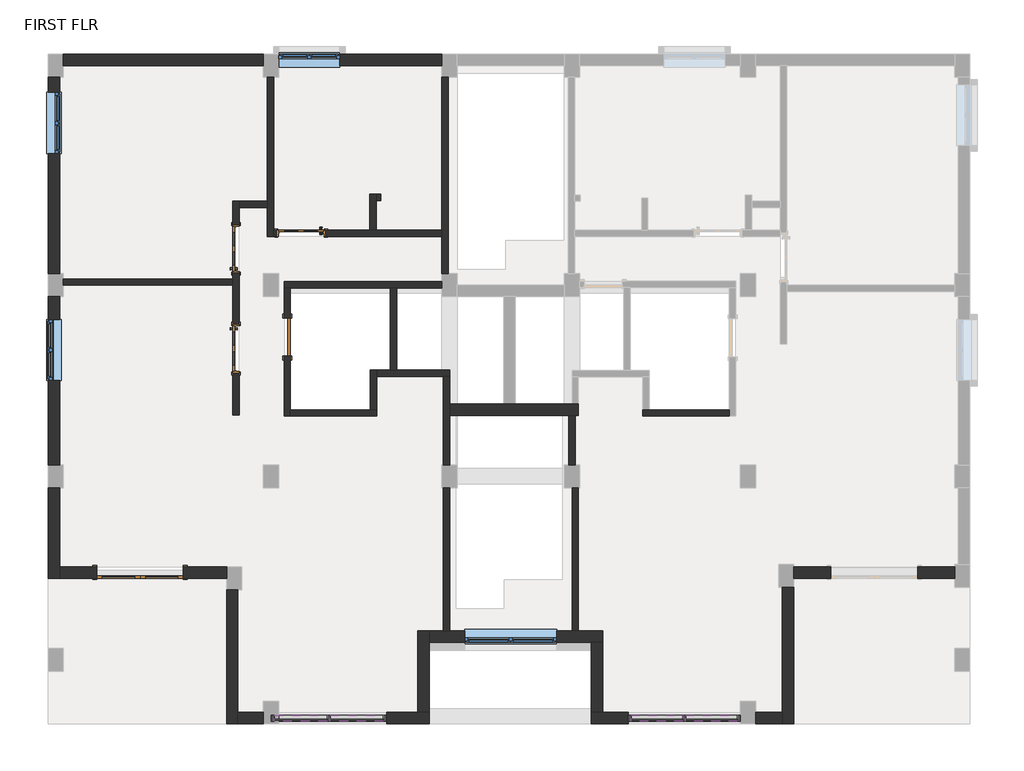
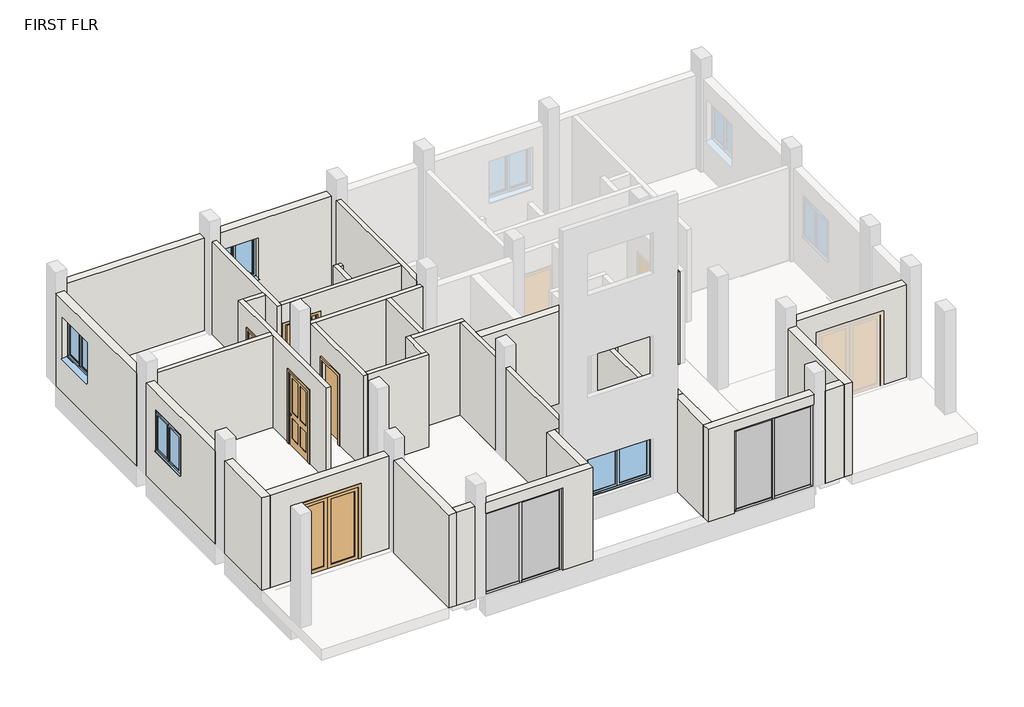
# One storey, part 1 of 3: 36 walls, 14 members, 5 doors, 4 plates, 4 windows.
"""IFC4 building model written with IfcOpenShell, lengths in millimetres."""

from ifc_helpers import new_model, si_unit, frame, origin, place, context, project, spatial, polyline, outline, extrude, faceted_brep, transform, mapped, element, save
from components import door_e52a3823, door_68a706ac, door_a823658d, door_1fe7f57d, member_a1c24a98, member_7fa39cca, member_f0fea5a5, member_ee409385, system_panel_glazed_8311221f, system_panel_glazed_a93c8db9, w2_0001_windows_4_x_4_9dec5fc7, w2_0001_window_4_x_6_83c3b52c

model = new_model("IFC4")

# Units and contexts
model_context = context("Model", 3, world=origin())
ifc_project = project(units=[si_unit("LENGTHUNIT", "METRE", prefix="MILLI")], contexts=[model_context])

# Site, building, storey
site = spatial("IfcSite", under=ifc_project)
building = spatial("IfcBuilding", under=site)
storey = spatial("IfcBuildingStorey", under=building, Name="FIRST FLR", Elevation=3352.8)

# Doors
placement = place(None, origin())
door_shape = door_e52a3823(model_context)
element("IfcDoor", 1, ObjectType="Door-Double-Glass : 68\" x 84\"", at=placement, inside=storey, context=model_context, shape_type="MappedRepresentation", body=[
    mapped(door_shape, transform((-7309.9981098, -11554.5807833, 3352.8), x_axis=(-1.0, 0.0, 0.0), y_axis=(0.0, -1.0, 0.0), z_axis=(0.0, 0.0, 1.0))),
])
door_2_shape = door_68a706ac(model_context)
element("IfcDoor", 2, ObjectType="Door-Interior-Single-4_Panel-Wood : 36\" x 84\"", at=placement, inside=storey, context=model_context, shape_type="MappedRepresentation", body=[
    mapped(door_2_shape, transform((-5402.1925798, -5105.3620333, 3352.8), x_axis=(0.0, 1.0, 0.0), y_axis=(-1.0, 0.0, 0.0), z_axis=(0.0, 0.0, 1.0))),
])
door_3_shape = door_a823658d(model_context)
element("IfcDoor", 3, ObjectType="Door-Interior-Single-4_Panel-Wood : 36\" x 84\"", at=placement, inside=storey, context=model_context, shape_type="MappedRepresentation", body=[
    mapped(door_3_shape, transform((-4103.6175798, -4789.1311634, 3352.8), x_axis=(-1.0, 0.0, 0.0), y_axis=(0.0, -1.0, 0.0), z_axis=(0.0, 0.0, 1.0))),
])
element("IfcDoor", 4, ObjectType="Door-Interior-Single-4_Panel-Wood : 36\" x 84\"", at=placement, inside=storey, context=model_context, shape_type="MappedRepresentation", body=[
    mapped(door_3_shape, transform((-5402.1925798, -7092.9120333, 3352.8), x_axis=(0.0, -1.0, 0.0), y_axis=(1.0, 0.0, 0.0), z_axis=(0.0, 0.0, 1.0))),
])
door_4_shape = door_1fe7f57d(model_context)
element("IfcDoor", 5, ObjectType="Single-Flush : 30\" x 80\"", at=placement, inside=storey, context=model_context, shape_type="MappedRepresentation", body=[
    mapped(door_4_shape, transform((-4379.0950401, -6863.7942903, 3352.8), x_axis=(0.0, -1.0, 0.0), y_axis=(1.0, 0.0, 0.0), z_axis=(0.0, 0.0, 1.0))),
])

# Members
member_shape = member_a1c24a98(model_context)
element("IfcMember", 6, ObjectType="Rectangular Mullion : 2.5\" x 5\" rectangular", at=placement, inside=storey, context=model_context, shape_type="MappedRepresentation", body=[
    mapped(member_shape, transform((2474.9824202, -14462.5402089, 5791.2), x_axis=(0.0, 0.0, 1.0), y_axis=(0.0, 1.0, 0.0), z_axis=(-1.0, 0.0, 0.0))),
])
element("IfcMember", 7, ObjectType="Rectangular Mullion : 2.5\" x 5\" rectangular", at=placement, inside=storey, context=model_context, shape_type="MappedRepresentation", body=[
    mapped(member_shape, transform((3560.8324202, -14462.5402089, 5791.2), x_axis=(0.0, 0.0, 1.0), y_axis=(0.0, 1.0, 0.0), z_axis=(-1.0, 0.0, 0.0))),
])
element("IfcMember", 8, ObjectType="Rectangular Mullion : 2.5\" x 5\" rectangular", at=placement, inside=storey, context=model_context, shape_type="MappedRepresentation", body=[
    mapped(member_shape, transform((4583.1824202, -14462.5402089, 3352.8), x_axis=(0.0, 0.0, -1.0), y_axis=(0.0, 1.0, 0.0), z_axis=(1.0, 0.0, 0.0))),
])
element("IfcMember", 9, ObjectType="Rectangular Mullion : 2.5\" x 5\" rectangular", at=placement, inside=storey, context=model_context, shape_type="MappedRepresentation", body=[
    mapped(member_shape, transform((3497.3324202, -14462.5402089, 3352.8), x_axis=(0.0, 0.0, -1.0), y_axis=(0.0, 1.0, 0.0), z_axis=(1.0, 0.0, 0.0))),
])
member_2_shape = member_7fa39cca(model_context)
element("IfcMember", 10, ObjectType="Rectangular Mullion : 2.5\" x 5\" rectangular", at=placement, inside=storey, context=model_context, shape_type="MappedRepresentation", body=[
    mapped(member_2_shape, transform((-4637.0175798, -14462.5402089, 5791.2), x_axis=(0.0, 0.0, 1.0), y_axis=(0.0, 1.0, 0.0), z_axis=(-1.0, 0.0, 0.0))),
])
element("IfcMember", 11, ObjectType="Rectangular Mullion : 2.5\" x 5\" rectangular", at=placement, inside=storey, context=model_context, shape_type="MappedRepresentation", body=[
    mapped(member_2_shape, transform((-3519.4175798, -14462.5402089, 5791.2), x_axis=(0.0, 0.0, 1.0), y_axis=(0.0, 1.0, 0.0), z_axis=(-1.0, 0.0, 0.0))),
])
element("IfcMember", 12, ObjectType="Rectangular Mullion : 2.5\" x 5\" rectangular", at=placement, inside=storey, context=model_context, shape_type="MappedRepresentation", body=[
    mapped(member_2_shape, transform((-2465.3175798, -14462.5402089, 3352.8), x_axis=(0.0, 0.0, -1.0), y_axis=(0.0, 1.0, 0.0), z_axis=(1.0, 0.0, 0.0))),
])
element("IfcMember", 13, ObjectType="Rectangular Mullion : 2.5\" x 5\" rectangular", at=placement, inside=storey, context=model_context, shape_type="MappedRepresentation", body=[
    mapped(member_2_shape, transform((-3582.9175798, -14462.5402089, 3352.8), x_axis=(0.0, 0.0, -1.0), y_axis=(0.0, 1.0, 0.0), z_axis=(1.0, 0.0, 0.0))),
])
member_3_shape = member_f0fea5a5(model_context)
element("IfcMember", 14, ObjectType="Rectangular Mullion : 2.5\" x 5\" rectangular", at=placement, inside=storey, context=model_context, shape_type="MappedRepresentation", body=[
    mapped(member_3_shape, transform((3529.0824202, -14462.5402089, 3352.8), x_axis=(-1.0, 0.0, 0.0), y_axis=(0.0, 1.0, 0.0), z_axis=(0.0, 0.0, -1.0))),
])
element("IfcMember", 15, ObjectType="Rectangular Mullion : 2.5\" x 5\" rectangular", at=placement, inside=storey, context=model_context, shape_type="MappedRepresentation", body=[
    mapped(member_3_shape, transform((-3551.1675798, -14462.5402089, 3352.8), x_axis=(-1.0, 0.0, 0.0), y_axis=(0.0, 1.0, 0.0), z_axis=(0.0, 0.0, -1.0))),
])
member_4_shape = member_ee409385(model_context)
element("IfcMember", 16, ObjectType="Rectangular Mullion : 2.5\" x 5\" rectangular", at=placement, inside=storey, context=model_context, shape_type="MappedRepresentation", body=[
    mapped(member_4_shape, transform((2411.4824202, -14462.5402089, 3352.8), x_axis=(-1.0, 0.0, 0.0), y_axis=(0.0, 1.0, 0.0), z_axis=(0.0, 0.0, -1.0))),
])
element("IfcMember", 17, ObjectType="Rectangular Mullion : 2.5\" x 5\" rectangular", at=placement, inside=storey, context=model_context, shape_type="MappedRepresentation", body=[
    mapped(member_4_shape, transform((-4700.5175798, -14462.5402089, 3352.8), x_axis=(-1.0, 0.0, 0.0), y_axis=(0.0, 1.0, 0.0), z_axis=(0.0, 0.0, -1.0))),
])
element("IfcMember", 18, ObjectType="Rectangular Mullion : 2.5\" x 5\" rectangular", at=placement, inside=storey, context=model_context, shape_type="MappedRepresentation", body=[
    mapped(member_4_shape, transform((4646.6824202, -14462.5402089, 5791.2), x_axis=(1.0, 0.0, 0.0), y_axis=(0.0, 1.0, 0.0), z_axis=(0.0, 0.0, 1.0))),
])
element("IfcMember", 19, ObjectType="Rectangular Mullion : 2.5\" x 5\" rectangular", at=placement, inside=storey, context=model_context, shape_type="MappedRepresentation", body=[
    mapped(member_4_shape, transform((-2401.8175798, -14462.5402089, 5791.2), x_axis=(1.0, 0.0, 0.0), y_axis=(0.0, 1.0, 0.0), z_axis=(0.0, 0.0, 1.0))),
])

# Plates
system_panel_glazed_shape = system_panel_glazed_8311221f(model_context)
element("IfcPlate", 20, ObjectType="System Panel : Glazed", at=placement, inside=storey, context=model_context, shape_type="MappedRepresentation", body=[
    mapped(system_panel_glazed_shape, transform((4072.0074202, -14462.5402089, 3416.3), x_axis=(-1.0, 0.0, 0.0), y_axis=(0.0, -1.0, 0.0), z_axis=(0.0, 0.0, 1.0))),
])
element("IfcPlate", 21, ObjectType="System Panel : Glazed", at=placement, inside=storey, context=model_context, shape_type="MappedRepresentation", body=[
    mapped(system_panel_glazed_shape, transform((2986.1574202, -14462.5402089, 3416.3), x_axis=(-1.0, 0.0, 0.0), y_axis=(0.0, -1.0, 0.0), z_axis=(0.0, 0.0, 1.0))),
])
system_panel_glazed_2_shape = system_panel_glazed_a93c8db9(model_context)
element("IfcPlate", 22, ObjectType="System Panel : Glazed", at=placement, inside=storey, context=model_context, shape_type="MappedRepresentation", body=[
    mapped(system_panel_glazed_2_shape, transform((-2992.3675798, -14462.5402089, 3416.3), x_axis=(-1.0, 0.0, 0.0), y_axis=(0.0, -1.0, 0.0), z_axis=(0.0, 0.0, 1.0))),
])
element("IfcPlate", 23, ObjectType="System Panel : Glazed", at=placement, inside=storey, context=model_context, shape_type="MappedRepresentation", body=[
    mapped(system_panel_glazed_2_shape, transform((-4109.9675798, -14462.5402089, 3416.3), x_axis=(-1.0, 0.0, 0.0), y_axis=(0.0, -1.0, 0.0), z_axis=(0.0, 0.0, 1.0))),
])

# Walls
element("IfcWall", 24, ObjectType="EXTERIOR WALL 9\"", at=placement, inside=storey, context=model_context, shape_type="SweptSolid", body=[
    extrude(outline(polyline([(-4852.9175798, -1452.2061634), (-8839.9786397, -1452.2061634), (-8839.9786397, -1223.6061634), (-4852.9175798, -1223.6061634), (-4852.9175798, -1452.2061634)])), frame((0.0, 0.0, 3352.8), z_axis=(0.0, 0.0, 1.0), x_axis=(1.0, 0.0, 0.0)), (0.0, 0.0, 1.0), 2743.2),
])
element("IfcWall", 25, ObjectType="EXTERIOR WALL 9\"", at=placement, inside=storey, context=model_context, shape_type="SweptSolid", body=[
    extrude(outline(polyline([(4352.8, -3328.9175798), (4352.8, -4548.1175798), (3352.8, -4548.1175798), (3352.8, -1296.9175798), (6096.0, -1296.9175798), (6096.0, -4548.1175798), (5572.0, -4548.1175798), (5572.0, -3328.9175798), (4352.8, -3328.9175798)])), frame((0.0, -1452.2061634, 0.0), z_axis=(0.0, 1.0, 0.0), x_axis=(0.0, 0.0, 1.0)), (0.0, 0.0, 1.0), 228.6),
])
element("IfcWall", 26, ObjectType="EXTERIOR WALL 9\"", at=placement, inside=storey, context=model_context, shape_type="SweptSolid", body=[
    extrude(outline(polyline([(-1680.8061634, 3352.8), (-5600.6620333, 3352.8), (-5600.6620333, 6096.0), (-1680.8061634, 6096.0), (-1680.8061634, 3352.8)]), holes=[polyline([(-3204.8061634, 4352.8), (-1985.6061634, 4352.8), (-1985.6061634, 5572.0), (-3204.8061634, 5572.0), (-3204.8061634, 4352.8)])]), frame((-9144.7786397, 0.0, 0.0), z_axis=(1.0, 0.0, 0.0), x_axis=(0.0, 1.0, 0.0)), (0.0, 0.0, 1.0), 228.6),
])
element("IfcWall", 27, ObjectType="EXTERIOR WALL 9\"", at=placement, inside=storey, context=model_context, shape_type="SweptSolid", body=[
    extrude(outline(polyline([(-6057.8620333, 3352.8), (-9410.6620333, 3352.8), (-9410.6620333, 6096.0), (-6057.8620333, 6096.0), (-6057.8620333, 3352.8)]), holes=[polyline([(-6515.0620333, 4352.8), (-6515.0620333, 5572.0), (-7734.2620333, 5572.0), (-7734.2620333, 4352.8), (-6515.0620333, 4352.8)])]), frame((-9144.7786397, 0.0, 0.0), z_axis=(1.0, 0.0, 0.0), x_axis=(0.0, 1.0, 0.0)), (0.0, 0.0, 1.0), 228.6),
])
element("IfcWall", 28, ObjectType="EXTERIOR WALL 9\"", at=placement, inside=storey, context=model_context, shape_type="Brep", body=[
    faceted_brep([(-9144.7786397, -9867.8620333, 3352.8), (-9144.7786397, -11671.2620333, 3352.8), (-9144.7786397, -11671.2620333, 6096.0), (-9144.7786397, -9867.8620333, 6096.0), (-8916.1786397, -9867.8620333, 3352.8), (-8916.1786397, -9867.8620333, 6096.0), (-8916.1786397, -11442.6620333, 6096.0), (-8916.1786397, -11671.2620333, 6096.0), (-8916.1786397, -11671.2620333, 3352.8), (-8916.1786397, -11442.6620333, 3352.8)], [[[0, 1, 2, 3]], [[4, 5, 6, 7, 8, 9]], [[1, 0, 4, 9, 8]], [[3, 2, 7, 6, 5]], [[0, 3, 5, 4]], [[2, 1, 8, 7]]]),
])
element("IfcWall", 29, ObjectType="EXTERIOR WALL 9\"", at=placement, inside=storey, context=model_context, shape_type="SweptSolid", body=[
    extrude(outline(polyline([(6096.0, -5589.5175798), (6096.0, -8916.1786397), (3352.8, -8916.1786397), (3352.8, -8173.5981098), (5486.4, -8173.5981098), (5486.4, -6446.3981098), (3352.8, -6446.3981098), (3352.8, -5589.5175798), (6096.0, -5589.5175798)])), frame((0.0, -11671.2620333, 0.0), z_axis=(0.0, 1.0, 0.0), x_axis=(0.0, 0.0, 1.0)), (0.0, 0.0, 1.0), 228.6),
])
element("IfcWall", 30, ObjectType="EXTERIOR WALL 9\"", at=placement, inside=storey, context=model_context, shape_type="SweptSolid", body=[
    extrude(outline(polyline([(6096.0, 5713.4824202), (3352.8, 5713.4824202), (3352.8, 6450.0824202), (5486.4, 6450.0824202), (5486.4, 8177.2824202), (3352.8, 8177.2824202), (3352.8, 8913.8824202), (6096.0, 8913.8824202), (6096.0, 5713.4824202)])), frame((0.0, -11671.2620333, 0.0), z_axis=(0.0, 1.0, 0.0), x_axis=(0.0, 0.0, 1.0)), (0.0, 0.0, 1.0), 228.6),
])
element("IfcWall", 31, ObjectType="EXTERIOR WALL 9\"", at=placement, inside=storey, context=model_context, shape_type="Brep", body=[
    faceted_brep([(5484.8824202, -11849.0620333, 3352.8), (5484.8824202, -14348.2402089, 3352.8), (5484.8824202, -14576.8402089, 3352.8), (5484.8824202, -14576.8402089, 6096.0), (5484.8824202, -14348.2402089, 6096.0), (5484.8824202, -11849.0620333, 6096.0), (5713.4824202, -11849.0620333, 3352.8), (5713.4824202, -11849.0620333, 6096.0), (5713.4824202, -14576.8402089, 6096.0), (5713.4824202, -14576.8402089, 3352.8)], [[[0, 1, 2, 3, 4, 5]], [[6, 7, 8, 9]], [[2, 1, 0, 6, 9]], [[5, 4, 3, 8, 7]], [[0, 5, 7, 6]], [[3, 2, 9, 8]]]),
])
element("IfcWall", 32, ObjectType="EXTERIOR WALL 9\"", at=placement, inside=storey, context=model_context, shape_type="SweptSolid", body=[
    extrude(outline(polyline([(5484.8824202, -14576.8402089), (4951.4824202, -14576.8402089), (4951.4824202, -14348.2402089), (5484.8824202, -14348.2402089), (5484.8824202, -14576.8402089)])), frame((0.0, 0.0, 3352.8), z_axis=(0.0, 0.0, 1.0), x_axis=(1.0, 0.0, 0.0)), (0.0, 0.0, 1.0), 2743.2),
])
element("IfcWall", 33, ObjectType="EXTERIOR WALL 9\"", at=placement, inside=storey, context=model_context, shape_type="Brep", body=[
    faceted_brep([(-5589.5175798, -11899.8620333, 3352.8), (-5589.5175798, -14576.8402089, 3352.8), (-5589.5175798, -14576.8402089, 6096.0), (-5589.5175798, -11899.8620333, 6096.0), (-5360.9175798, -11899.8620333, 3352.8), (-5360.9175798, -11899.8620333, 6096.0), (-5360.9175798, -14348.2402089, 6096.0), (-5360.9175798, -14576.8402089, 6096.0), (-5360.9175798, -14576.8402089, 3352.8), (-5360.9175798, -14348.2402089, 3352.8)], [[[0, 1, 2, 3]], [[4, 5, 6, 7, 8, 9]], [[1, 0, 4, 9, 8]], [[3, 2, 7, 6, 5]], [[0, 3, 5, 4]], [[2, 1, 8, 7]]]),
])
element("IfcWall", 34, ObjectType="EXTERIOR WALL 9\"", at=placement, inside=storey, context=model_context, shape_type="SweptSolid", body=[
    extrude(outline(polyline([(-5360.9175798, -14348.2402089), (-4852.9175798, -14348.2402089), (-4852.9175798, -14576.8402089), (-5360.9175798, -14576.8402089), (-5360.9175798, -14348.2402089)])), frame((0.0, 0.0, 3352.8), z_axis=(0.0, 0.0, 1.0), x_axis=(1.0, 0.0, 0.0)), (0.0, 0.0, 1.0), 2743.2),
])
element("IfcWall", 35, ObjectType="EXTERIOR WALL 9\"", at=placement, inside=storey, context=model_context, shape_type="Brep", body=[
    faceted_brep([(1674.8824202, -14348.2402089, 6096.0), (1903.4824202, -14348.2402089, 6096.0), (4646.6824202, -14348.2402089, 6096.0), (4646.6824202, -14348.2402089, 5791.2), (2411.4824202, -14348.2402089, 5791.2), (2411.4824202, -14348.2402089, 3352.8), (1903.4824202, -14348.2402089, 3352.8), (1674.8824202, -14348.2402089, 3352.8), (4646.6824202, -14576.8402089, 6096.0), (1674.8824202, -14576.8402089, 6096.0), (1674.8824202, -14576.8402089, 3352.8), (2411.4824202, -14576.8402089, 3352.8), (2411.4824202, -14576.8402089, 5791.2), (4646.6824202, -14576.8402089, 5791.2)], [[[0, 1, 2, 3, 4, 5, 6, 7]], [[8, 9, 10, 11, 12, 13]], [[10, 7, 6, 5, 11]], [[2, 1, 0, 9, 8]], [[2, 8, 13, 3]], [[0, 7, 10, 9]], [[4, 12, 11, 5]], [[12, 4, 3, 13]]]),
])
element("IfcWall", 36, ObjectType="EXTERIOR WALL 9\"", at=placement, inside=storey, context=model_context, shape_type="Brep", body=[
    faceted_brep([(-1550.9175798, -14576.8402089, 6096.0), (-4548.1175798, -14576.8402089, 6096.0), (-4548.1175798, -14576.8402089, 5791.2), (-2401.8175798, -14576.8402089, 5791.2), (-2401.8175798, -14576.8402089, 3352.8), (-1550.9175798, -14576.8402089, 3352.8), (-4548.1175798, -14348.2402089, 6096.0), (-1779.5175798, -14348.2402089, 6096.0), (-1550.9175798, -14348.2402089, 6096.0), (-1550.9175798, -14348.2402089, 3352.8), (-1779.5175798, -14348.2402089, 3352.8), (-2401.8175798, -14348.2402089, 3352.8), (-2401.8175798, -14348.2402089, 5791.2), (-4548.1175798, -14348.2402089, 5791.2)], [[[0, 1, 2, 3, 4, 5]], [[6, 7, 8, 9, 10, 11, 12, 13]], [[9, 5, 4, 11, 10]], [[1, 0, 8, 7, 6]], [[1, 6, 13, 2]], [[0, 5, 9, 8]], [[3, 12, 11, 4]], [[12, 3, 2, 13]]]),
])
element("IfcWall", 37, ObjectType="EXTERIOR WALL 9\"", at=placement, inside=storey, context=model_context, shape_type="Brep", body=[
    faceted_brep([(-1550.9175798, -14348.2402089, 3352.8), (-1550.9175798, -12951.2402089, 3352.8), (-1550.9175798, -12722.6402089, 3352.8), (-1550.9175798, -12722.6402089, 6096.0), (-1550.9175798, -12951.2402089, 6096.0), (-1550.9175798, -14348.2402089, 6096.0), (-1779.5175798, -14348.2402089, 3352.8), (-1779.5175798, -14348.2402089, 6096.0), (-1779.5175798, -12722.6402089, 6096.0), (-1779.5175798, -12722.6402089, 3352.8)], [[[0, 1, 2, 3, 4, 5]], [[6, 7, 8, 9]], [[2, 1, 0, 6, 9]], [[5, 4, 3, 8, 7]], [[0, 5, 7, 6]], [[3, 2, 9, 8]]]),
])
element("IfcWall", 38, ObjectType="EXTERIOR WALL 9\"", at=placement, inside=storey, context=model_context, shape_type="Brep", body=[
    faceted_brep([(-1550.9175798, -12951.2402089, 3352.8), (1674.8824202, -12951.2402089, 3352.8), (1903.4824202, -12951.2402089, 3352.8), (1903.4824202, -12951.2402089, 6096.0), (1674.8824202, -12951.2402089, 6096.0), (-1550.9175798, -12951.2402089, 6096.0), (-839.7175798, -12951.2402089, 3962.4), (-839.7175798, -12951.2402089, 5181.6), (989.0824202, -12951.2402089, 5181.6), (989.0824202, -12951.2402089, 3962.4), (-1550.9175798, -12722.6402089, 3352.8), (-1550.9175798, -12722.6402089, 6096.0), (-1271.5175798, -12722.6402089, 6096.0), (-1144.5175798, -12722.6402089, 6096.0), (1293.8824202, -12722.6402089, 6096.0), (1420.8824202, -12722.6402089, 6096.0), (1903.4824202, -12722.6402089, 6096.0), (1903.4824202, -12722.6402089, 3352.8), (1420.8824202, -12722.6402089, 3352.8), (1293.8824202, -12722.6402089, 3352.8), (-1144.5175798, -12722.6402089, 3352.8), (-1271.5175798, -12722.6402089, 3352.8), (-839.7175798, -12722.6402089, 3962.4), (989.0824202, -12722.6402089, 3962.4), (989.0824202, -12722.6402089, 5181.6), (-839.7175798, -12722.6402089, 5181.6)], [[[0, 1, 2, 3, 4, 5], [6, 7, 8, 9]], [[10, 11, 12, 13, 14, 15, 16, 17, 18, 19, 20, 21], [22, 23, 24, 25]], [[2, 1, 0, 10, 21, 20, 19, 18, 17]], [[5, 4, 3, 16, 15, 14, 13, 12, 11]], [[0, 5, 11, 10]], [[3, 2, 17, 16]], [[7, 6, 22, 25]], [[8, 7, 25, 24]], [[9, 8, 24, 23]], [[6, 9, 23, 22]]]),
])
element("IfcWall", 39, ObjectType="EXTERIOR WALL 9\"", at=placement, inside=storey, context=model_context, shape_type="SweptSolid", body=[
    extrude(outline(polyline([(1674.8824202, -14348.2402089), (1674.8824202, -12951.2402089), (1903.4824202, -12951.2402089), (1903.4824202, -14348.2402089), (1674.8824202, -14348.2402089)])), frame((0.0, 0.0, 3352.8), z_axis=(0.0, 0.0, 1.0), x_axis=(1.0, 0.0, 0.0)), (0.0, 0.0, 1.0), 2743.2),
])
element("IfcWall", 40, ObjectType="EXTERIOR WALL 9\"", at=placement, inside=storey, context=model_context, shape_type="Brep", body=[
    faceted_brep([(-1144.5175798, -8426.4120333, 3352.8), (1230.3824202, -8426.4120333, 3352.8), (1357.3824202, -8426.4120333, 3352.8), (1420.8824202, -8426.4120333, 3352.8), (1420.8824202, -8426.4120333, 6096.0), (1357.3824202, -8426.4120333, 6096.0), (1230.3824202, -8426.4120333, 6096.0), (-1144.5175798, -8426.4120333, 6096.0), (-1144.5175798, -8197.8120333, 3352.8), (-1144.5175798, -8197.8120333, 6096.0), (-65.0175798, -8197.8120333, 6096.0), (163.5824202, -8197.8120333, 6096.0), (1293.8824202, -8197.8120333, 6096.0), (1420.8824202, -8197.8120333, 6096.0), (1420.8824202, -8197.8120333, 3352.8), (1293.8824202, -8197.8120333, 3352.8), (163.5824202, -8197.8120333, 3352.8), (-65.0175798, -8197.8120333, 3352.8)], [[[0, 1, 2, 3, 4, 5, 6, 7]], [[8, 9, 10, 11, 12, 13, 14, 15, 16, 17]], [[3, 2, 1, 0, 8, 17, 16, 15, 14]], [[7, 6, 5, 4, 13, 12, 11, 10, 9]], [[0, 7, 9, 8]], [[4, 3, 14, 13]]]),
])
element("IfcWall", 41, ObjectType="INTERIOR WALL 5\"", at=placement, inside=storey, context=model_context, shape_type="SweptSolid", body=[
    extrude(outline(polyline([(-5462.5175798, -5829.2620333), (-8839.9786397, -5829.2620333), (-8839.9786397, -5702.2620333), (-5462.5175798, -5702.2620333), (-5462.5175798, -5829.2620333)])), frame((0.0, 0.0, 3352.8), z_axis=(0.0, 0.0, 1.0), x_axis=(1.0, 0.0, 0.0)), (0.0, 0.0, 1.0), 2743.2),
])
element("IfcWall", 42, ObjectType="INTERIOR WALL 5\"", at=placement, inside=storey, context=model_context, shape_type="Brep", body=[
    faceted_brep([(-5462.5175798, -8420.0620333, 3352.8), (-5462.5175798, -8420.0620333, 6096.0), (-5462.5175798, -5829.2620333, 6096.0), (-5462.5175798, -5702.2620333, 6096.0), (-5462.5175798, -4153.3104011, 6096.0), (-5462.5175798, -4153.3104011, 3352.8), (-5462.5175798, -4622.7620333, 3352.8), (-5462.5175798, -4622.7620333, 5511.8), (-5462.5175798, -5587.9620333, 5511.8), (-5462.5175798, -5587.9620333, 3352.8), (-5462.5175798, -5702.2620333, 3352.8), (-5462.5175798, -5829.2620333, 3352.8), (-5462.5175798, -6610.3120333, 3352.8), (-5462.5175798, -6610.3120333, 5511.8), (-5462.5175798, -7575.5120333, 5511.8), (-5462.5175798, -7575.5120333, 3352.8), (-5335.5175798, -8420.0620333, 6096.0), (-5335.5175798, -8420.0620333, 3352.8), (-5335.5175798, -7575.5120333, 3352.8), (-5335.5175798, -7575.5120333, 5511.8), (-5335.5175798, -6610.3120333, 5511.8), (-5335.5175798, -6610.3120333, 3352.8), (-5335.5175798, -5587.9620333, 3352.8), (-5335.5175798, -5587.9620333, 5511.8), (-5335.5175798, -4622.7620333, 5511.8), (-5335.5175798, -4622.7620333, 3352.8), (-5335.5175798, -4280.3104011, 3352.8), (-5335.5175798, -4153.3104011, 3352.8), (-5335.5175798, -4153.3104011, 6096.0), (-5335.5175798, -4280.3104011, 6096.0)], [[[0, 1, 2, 3, 4, 5, 6, 7, 8, 9, 10, 11, 12, 13, 14, 15]], [[16, 17, 18, 19, 20, 21, 22, 23, 24, 25, 26, 27, 28, 29]], [[17, 0, 15, 18]], [[5, 27, 26, 25, 6]], [[9, 22, 21, 12, 11, 10]], [[1, 0, 17, 16]], [[4, 3, 2, 1, 16, 29, 28]], [[5, 4, 28, 27]], [[24, 7, 6, 25]], [[7, 24, 23, 8]], [[8, 23, 22, 9]], [[14, 19, 18, 15]], [[19, 14, 13, 20]], [[20, 13, 12, 21]]]),
])
element("IfcWall", 43, ObjectType="INTERIOR WALL 5\"", at=placement, inside=storey, context=model_context, shape_type="SweptSolid", body=[
    extrude(outline(polyline([(-4776.7175798, -4280.3104011), (-5335.5175798, -4280.3104011), (-5335.5175798, -4153.3104011), (-4776.7175798, -4153.3104011), (-4776.7175798, -4280.3104011)])), frame((0.0, 0.0, 3352.8), z_axis=(0.0, 0.0, 1.0), x_axis=(1.0, 0.0, 0.0)), (0.0, 0.0, 1.0), 2743.2),
])
element("IfcWall", 44, ObjectType="INTERIOR WALL 5\"", at=placement, inside=storey, context=model_context, shape_type="Brep", body=[
    faceted_brep([(-4776.7175798, -1680.8061634, 3352.8), (-4776.7175798, -4153.3104011, 3352.8), (-4776.7175798, -4280.3104011, 3352.8), (-4776.7175798, -4855.8061634, 3352.8), (-4776.7175798, -4855.8061634, 6096.0), (-4776.7175798, -4280.3104011, 6096.0), (-4776.7175798, -4153.3104011, 6096.0), (-4776.7175798, -1680.8061634, 6096.0), (-4649.7175798, -1680.8061634, 3352.8), (-4649.7175798, -1680.8061634, 6096.0), (-4649.7175798, -4728.8061634, 6096.0), (-4649.7175798, -4855.8061634, 6096.0), (-4649.7175798, -4855.8061634, 3352.8), (-4649.7175798, -4728.8061634, 3352.8)], [[[0, 1, 2, 3, 4, 5, 6, 7]], [[8, 9, 10, 11, 12, 13]], [[3, 2, 1, 0, 8, 13, 12]], [[7, 6, 5, 4, 11, 10, 9]], [[0, 7, 9, 8]], [[4, 3, 12, 11]]]),
])
element("IfcWall", 45, ObjectType="INTERIOR WALL 5\"", at=placement, inside=storey, context=model_context, shape_type="Brep", body=[
    faceted_brep([(-1296.9175798, -4855.8061634, 6096.0), (-4649.7175798, -4855.8061634, 6096.0), (-4649.7175798, -4855.8061634, 3352.8), (-4586.2175798, -4855.8061634, 3352.8), (-4586.2175798, -4855.8061634, 5511.8), (-3621.0175798, -4855.8061634, 5511.8), (-3621.0175798, -4855.8061634, 3352.8), (-1296.9175798, -4855.8061634, 3352.8), (-4649.7175798, -4728.8061634, 6096.0), (-2732.0175798, -4728.8061634, 6096.0), (-2605.0175798, -4728.8061634, 6096.0), (-1296.9175798, -4728.8061634, 6096.0), (-1296.9175798, -4728.8061634, 3352.8), (-2605.0175798, -4728.8061634, 3352.8), (-2732.0175798, -4728.8061634, 3352.8), (-3621.0175798, -4728.8061634, 3352.8), (-3621.0175798, -4728.8061634, 5511.8), (-4586.2175798, -4728.8061634, 5511.8), (-4586.2175798, -4728.8061634, 3352.8), (-4649.7175798, -4728.8061634, 3352.8)], [[[0, 1, 2, 3, 4, 5, 6, 7]], [[8, 9, 10, 11, 12, 13, 14, 15, 16, 17, 18, 19]], [[2, 19, 18, 3]], [[12, 7, 6, 15, 14, 13]], [[1, 0, 11, 10, 9, 8]], [[2, 1, 8, 19]], [[0, 7, 12, 11]], [[17, 4, 3, 18]], [[4, 17, 16, 5]], [[5, 16, 15, 6]]]),
])
element("IfcWall", 46, ObjectType="INTERIOR WALL 5\"", at=placement, inside=storey, context=model_context, shape_type="Brep", body=[
    faceted_brep([(-1296.9175798, -1680.8061634, 3352.8), (-1296.9175798, -4728.8061634, 3352.8), (-1296.9175798, -4855.8061634, 3352.8), (-1296.9175798, -5600.6620333, 3352.8), (-1296.9175798, -5600.6620333, 6096.0), (-1296.9175798, -4855.8061634, 6096.0), (-1296.9175798, -4728.8061634, 6096.0), (-1296.9175798, -1680.8061634, 6096.0), (-1169.9175798, -1680.8061634, 3352.8), (-1169.9175798, -1680.8061634, 6096.0), (-1169.9175798, -5600.6620333, 6096.0), (-1169.9175798, -5600.6620333, 3352.8)], [[[0, 1, 2, 3, 4, 5, 6, 7]], [[8, 9, 10, 11]], [[3, 2, 1, 0, 8, 11]], [[4, 3, 11, 10]], [[7, 6, 5, 4, 10, 9]], [[0, 7, 9, 8]]]),
])
element("IfcWall", 47, ObjectType="INTERIOR WALL 5\"", at=placement, inside=storey, context=model_context, shape_type="Brep", body=[
    faceted_brep([(-2605.0175798, -4728.8061634, 3352.8), (-2605.0175798, -4144.6061634, 3352.8), (-2605.0175798, -4017.6061634, 3352.8), (-2605.0175798, -4017.6061634, 6096.0), (-2605.0175798, -4144.6061634, 6096.0), (-2605.0175798, -4728.8061634, 6096.0), (-2732.0175798, -4728.8061634, 3352.8), (-2732.0175798, -4728.8061634, 6096.0), (-2732.0175798, -4017.6061634, 6096.0), (-2732.0175798, -4017.6061634, 3352.8)], [[[0, 1, 2, 3, 4, 5]], [[6, 7, 8, 9]], [[2, 1, 0, 6, 9]], [[5, 4, 3, 8, 7]], [[0, 5, 7, 6]], [[3, 2, 9, 8]]]),
])
element("IfcWall", 48, ObjectType="INTERIOR WALL 5\"", at=placement, inside=storey, context=model_context, shape_type="SweptSolid", body=[
    extrude(outline(polyline([(-2605.0175798, -4017.6061634), (-2516.1175798, -4017.6061634), (-2516.1175798, -4144.6061634), (-2605.0175798, -4144.6061634), (-2605.0175798, -4017.6061634)])), frame((0.0, 0.0, 3352.8), z_axis=(0.0, 0.0, 1.0), x_axis=(1.0, 0.0, 0.0)), (0.0, 0.0, 1.0), 2743.2),
])
element("IfcWall", 49, ObjectType="INTERIOR WALL 5\"", at=placement, inside=storey, context=model_context, shape_type="Brep", body=[
    faceted_brep([(-4442.5950401, -5885.8942903, 3352.8), (-4315.5950401, -5885.8942903, 3352.8), (-2325.6175798, -5885.8942903, 3352.8), (-2198.6175798, -5885.8942903, 3352.8), (-1296.9175798, -5885.8942903, 3352.8), (-1296.9175798, -5885.8942903, 6096.0), (-2198.6175798, -5885.8942903, 6096.0), (-2325.6175798, -5885.8942903, 6096.0), (-4315.5950401, -5885.8942903, 6096.0), (-4442.5950401, -5885.8942903, 6096.0), (-4442.5950401, -5758.8942903, 3352.8), (-4442.5950401, -5758.8942903, 6096.0), (-1296.9175798, -5758.8942903, 6096.0), (-1296.9175798, -5758.8942903, 3352.8)], [[[0, 1, 2, 3, 4, 5, 6, 7, 8, 9]], [[10, 11, 12, 13]], [[4, 3, 2, 1, 0, 10, 13]], [[5, 4, 13, 12]], [[9, 8, 7, 6, 5, 12, 11]], [[0, 9, 11, 10]]]),
])
element("IfcWall", 50, ObjectType="INTERIOR WALL 5\"", at=placement, inside=storey, context=model_context, shape_type="Brep", body=[
    faceted_brep([(-4442.5950401, -7244.7942903, 5384.8), (-4442.5950401, -7244.7942903, 3352.8), (-4442.5950401, -8439.1120333, 3352.8), (-4442.5950401, -8439.1120333, 6096.0), (-4442.5950401, -5885.8942903, 6096.0), (-4442.5950401, -5885.8942903, 3352.8), (-4442.5950401, -6482.7942903, 3352.8), (-4442.5950401, -6482.7942903, 5384.8), (-4315.5950401, -8439.1120333, 3352.8), (-4315.5950401, -8312.1120333, 3352.8), (-4315.5950401, -7244.7942903, 3352.8), (-4315.5950401, -7244.7942903, 5384.8), (-4315.5950401, -6482.7942903, 5384.8), (-4315.5950401, -6482.7942903, 3352.8), (-4315.5950401, -5885.8942903, 3352.8), (-4315.5950401, -5885.8942903, 6096.0), (-4315.5950401, -8312.1120333, 6096.0), (-4315.5950401, -8439.1120333, 6096.0)], [[[0, 1, 2, 3, 4, 5, 6, 7]], [[8, 9, 10, 11, 12, 13, 14, 15, 16, 17]], [[6, 5, 14, 13]], [[2, 1, 10, 9, 8]], [[4, 3, 17, 16, 15]], [[5, 4, 15, 14]], [[3, 2, 8, 17]], [[11, 10, 1, 0]], [[12, 11, 0, 7]], [[13, 12, 7, 6]]]),
])
element("IfcWall", 51, ObjectType="INTERIOR WALL 5\"", at=placement, inside=storey, context=model_context, shape_type="Brep", body=[
    faceted_brep([(-4315.5950401, -8439.1120333, 3352.8), (-2601.0950401, -8439.1120333, 3352.8), (-2601.0950401, -8439.1120333, 6096.0), (-4315.5950401, -8439.1120333, 6096.0), (-4315.5950401, -8312.1120333, 3352.8), (-4315.5950401, -8312.1120333, 6096.0), (-2728.0950401, -8312.1120333, 6096.0), (-2601.0950401, -8312.1120333, 6096.0), (-2601.0950401, -8312.1120333, 3352.8), (-2728.0950401, -8312.1120333, 3352.8)], [[[0, 1, 2, 3]], [[4, 5, 6, 7, 8, 9]], [[1, 0, 4, 9, 8]], [[3, 2, 7, 6, 5]], [[0, 3, 5, 4]], [[2, 1, 8, 7]]]),
])
element("IfcWall", 52, ObjectType="INTERIOR WALL 5\"", at=placement, inside=storey, context=model_context, shape_type="Brep", body=[
    faceted_brep([(-2601.0950401, -8312.1120333, 3352.8), (-2601.0950401, -7651.7120333, 3352.8), (-2601.0950401, -7524.7120333, 3352.8), (-2601.0950401, -7524.7120333, 6096.0), (-2601.0950401, -7651.7120333, 6096.0), (-2601.0950401, -8312.1120333, 6096.0), (-2728.0950401, -8312.1120333, 3352.8), (-2728.0950401, -8312.1120333, 6096.0), (-2728.0950401, -7524.7120333, 6096.0), (-2728.0950401, -7524.7120333, 3352.8)], [[[0, 1, 2, 3, 4, 5]], [[6, 7, 8, 9]], [[2, 1, 0, 6, 9]], [[5, 4, 3, 8, 7]], [[0, 5, 7, 6]], [[3, 2, 9, 8]]]),
])
element("IfcWall", 53, ObjectType="INTERIOR WALL 5\"", at=placement, inside=storey, context=model_context, shape_type="Brep", body=[
    faceted_brep([(-2601.0950401, -7651.7120333, 3352.8), (-1271.5175798, -7651.7120333, 3352.8), (-1144.5175798, -7651.7120333, 3352.8), (-1144.5175798, -7651.7120333, 6096.0), (-1271.5175798, -7651.7120333, 6096.0), (-2601.0950401, -7651.7120333, 6096.0), (-2601.0950401, -7524.7120333, 3352.8), (-2601.0950401, -7524.7120333, 6096.0), (-2325.6175798, -7524.7120333, 6096.0), (-2198.6175798, -7524.7120333, 6096.0), (-1144.5175798, -7524.7120333, 6096.0), (-1144.5175798, -7524.7120333, 3352.8), (-2198.6175798, -7524.7120333, 3352.8), (-2325.6175798, -7524.7120333, 3352.8)], [[[0, 1, 2, 3, 4, 5]], [[6, 7, 8, 9, 10, 11, 12, 13]], [[2, 1, 0, 6, 13, 12, 11]], [[5, 4, 3, 10, 9, 8, 7]], [[0, 5, 7, 6]], [[3, 2, 11, 10]]]),
])
element("IfcWall", 54, ObjectType="INTERIOR WALL 5\"", at=placement, inside=storey, context=model_context, shape_type="SweptSolid", body=[
    extrude(outline(polyline([(-2325.6175798, -7524.7120333), (-2325.6175798, -5885.8942903), (-2198.6175798, -5885.8942903), (-2198.6175798, -7524.7120333), (-2325.6175798, -7524.7120333)])), frame((0.0, 0.0, 3352.8), z_axis=(0.0, 0.0, 1.0), x_axis=(1.0, 0.0, 0.0)), (0.0, 0.0, 1.0), 2743.2),
])
element("IfcWall", 55, ObjectType="INTERIOR WALL 5\"", at=placement, inside=storey, context=model_context, shape_type="Brep", body=[
    faceted_brep([(-1271.5175798, -7651.7120333, 3352.8), (-1271.5175798, -9417.0120333, 3352.8), (-1271.5175798, -9417.0120333, 6096.0), (-1271.5175798, -7651.7120333, 6096.0), (-1144.5175798, -7651.7120333, 3352.8), (-1144.5175798, -7651.7120333, 6096.0), (-1144.5175798, -8197.8120333, 6096.0), (-1144.5175798, -8426.4120333, 6096.0), (-1144.5175798, -9417.0120333, 6096.0), (-1144.5175798, -9417.0120333, 3352.8), (-1144.5175798, -8426.4120333, 3352.8), (-1144.5175798, -8197.8120333, 3352.8)], [[[0, 1, 2, 3]], [[4, 5, 6, 7, 8, 9, 10, 11]], [[1, 0, 4, 11, 10, 9]], [[2, 1, 9, 8]], [[3, 2, 8, 7, 6, 5]], [[0, 3, 5, 4]]]),
])
element("IfcWall", 56, ObjectType="INTERIOR WALL 5\"", at=placement, inside=storey, context=model_context, shape_type="Brep", body=[
    faceted_brep([(4430.7824202, -8312.7691591, 3352.8), (2830.5824202, -8312.7691591, 3352.8), (2703.5824202, -8312.7691591, 3352.8), (2703.5824202, -8312.7691591, 6096.0), (2830.5824202, -8312.7691591, 6096.0), (4430.7824202, -8312.7691591, 6096.0), (4430.7824202, -8439.7691591, 3352.8), (4430.7824202, -8439.7691591, 6096.0), (2703.5824202, -8439.7691591, 6096.0), (2703.5824202, -8439.7691591, 3352.8)], [[[0, 1, 2, 3, 4, 5]], [[6, 7, 8, 9]], [[2, 1, 0, 6, 9]], [[5, 4, 3, 8, 7]], [[0, 5, 7, 6]], [[3, 2, 9, 8]]]),
])
element("IfcWall", 57, ObjectType="INTERIOR WALL 5\"", at=placement, inside=storey, context=model_context, shape_type="SweptSolid", body=[
    extrude(outline(polyline([(-1271.5175798, -12722.6402089), (-1271.5175798, -9867.8620333), (-1144.5175798, -9867.8620333), (-1144.5175798, -12722.6402089), (-1271.5175798, -12722.6402089)])), frame((0.0, 0.0, 3352.8), z_axis=(0.0, 0.0, 1.0), x_axis=(1.0, 0.0, 0.0)), (0.0, 0.0, 1.0), 2743.2),
])
element("IfcWall", 58, ObjectType="INTERIOR WALL 5\"", at=placement, inside=storey, context=model_context, shape_type="SweptSolid", body=[
    extrude(outline(polyline([(1293.8824202, -12722.6402089), (1293.8824202, -9867.8620333), (1420.8824202, -9867.8620333), (1420.8824202, -12722.6402089), (1293.8824202, -12722.6402089)])), frame((0.0, 0.0, 3352.8), z_axis=(0.0, 0.0, 1.0), x_axis=(1.0, 0.0, 0.0)), (0.0, 0.0, 1.0), 2743.2),
])
element("IfcWall", 59, ObjectType="INTERIOR WALL 5\"", at=placement, inside=storey, context=model_context, shape_type="SweptSolid", body=[
    extrude(outline(polyline([(1357.3824202, -8426.4120333), (1357.3824202, -9410.6620333), (1230.3824202, -9410.6620333), (1230.3824202, -8426.4120333), (1357.3824202, -8426.4120333)])), frame((0.0, 0.0, 3352.8), z_axis=(0.0, 0.0, 1.0), x_axis=(1.0, 0.0, 0.0)), (0.0, 0.0, 1.0), 2743.2),
])

# Windows
w2_0001_windows_4_x_4_shape = w2_0001_windows_4_x_4_9dec5fc7(model_context)
element("IfcWindow", 60, ObjectType="w2.0001 : WINDOWS 4' X 4'", at=placement, inside=storey, context=model_context, shape_type="MappedRepresentation", body=[
    mapped(w2_0001_windows_4_x_4_shape, transform((-9030.4786397, -2595.2061634, 3352.8), x_axis=(0.0, 1.0, 0.0), y_axis=(-1.0, 0.0, 0.0), z_axis=(0.0, 0.0, 1.0))),
])
element("IfcWindow", 61, ObjectType="w2.0001 : WINDOWS 4' X 4'", at=placement, inside=storey, context=model_context, shape_type="MappedRepresentation", body=[
    mapped(w2_0001_windows_4_x_4_shape, transform((-9030.4786397, -7124.6620333, 3352.8), x_axis=(0.0, -1.0, 0.0), y_axis=(1.0, 0.0, 0.0), z_axis=(0.0, 0.0, 1.0))),
])
element("IfcWindow", 62, ObjectType="w2.0001 : WINDOWS 4' X 4'", at=placement, inside=storey, context=model_context, shape_type="MappedRepresentation", body=[
    mapped(w2_0001_windows_4_x_4_shape, transform((-3938.5175798, -1337.9061634, 3352.8), x_axis=(-1.0, 0.0, 0.0), y_axis=(0.0, -1.0, 0.0), z_axis=(0.0, 0.0, 1.0))),
])
w2_0001_window_4_x_6_shape = w2_0001_window_4_x_6_83c3b52c(model_context)
element("IfcWindow", 63, ObjectType="w2.0001 : window 4' x 6'", at=placement, inside=storey, context=model_context, shape_type="MappedRepresentation", body=[
    mapped(w2_0001_window_4_x_6_shape, transform((74.6824202, -12836.9402089, 2962.4), x_axis=(1.0, 0.0, 0.0), y_axis=(0.0, 1.0, 0.0), z_axis=(0.0, 0.0, 1.0))),
])

save(model, "model.ifc")

# Revit data of these elements
# Type "Door-Double-Glass : 68\" x 84\""
#   Type Mark = "11"
#   Construction Type Id = "opn-d45"
#   Assembly Code = "C1020"
#   Analytic Construction = "Wood frame, double glass door "
#   W = 2' - 10"
#   Thickness = 0' - 2"
#   Thermal Resistance (R) = 1.8150 (h·ft²·°F)/BTU
#   Swing Angle [instance default] = 90.00°
#   Heat Transfer Coefficient (U) = 0.5510 BTU/(h·ft²·°F)
#   Height = 7' - 0"
#   Bottom Rail = 0' - 4"
#   Top Rail = 0' - 4"
#   Stiles = 0' - 4"
#   Trim Projection = 0' - 1"
#   Trim Width = 0' - 3"
#   Width = 5' - 8"
#   Define Thermal Properties by = 1
#   Glazing = Glass
#   Panel Material = Wood - Birch - Solid Stained Light Low Gloss
#   Trim Material = Paint - Sienna
#   Visual Light Transmittance = 0
#   Solar Heat Gain Coefficient = 0
#   Function = (empty or 0)
#   Wall Closure = (empty or 0)
# Type "Door-Interior-Single-4_Panel-Wood : 36\" x 84\""
#   Type Mark = "9"
#   Assembly Code = "C1020300"
#   Analytic Construction = "Wooden"
#   Top Rail = 0' - 4 11/16"
#   Thickness = 0' - 1 3/8"
#   Thermal Resistance (R) = 2.5876 (h·ft²·°F)/BTU
#   Swing Angle [instance default] = 90.00°
#   Stiles = 0' - 4 3/4"
#   Rough Width = 3' - 2"
#   Rough Height = 7' - 1"
#   Mullion = 0' - 4 1/2"
#   Lock Rail = 0' - 7 1/2"
#   Height = 7' - 0"
#   Width = 3' - 0"
#   Heat Transfer Coefficient (U) = 0.3865 BTU/(h·ft²·°F)
#   Bottom Rail = 0' - 9 1/8"
#   Trim Material = Cherry
#   Panel Material = Cherry
#   Frame Material = Cherry
#   Door Handle Material = Aluminum
#   Visual Light Transmittance = 0
#   Solar Heat Gain Coefficient = 0
#   Wall Closure = (empty or 0)
#   Function = (empty or 0)
# Type "Single-Flush : 30\" x 80\""
#   Type Mark = "5"
#   Construction Type Id = "MDOOR"
#   Assembly Code = "C1020"
#   Analytic Construction = "Metal"
#   Thickness = 0' - 2"
#   Heat Transfer Coefficient (U) = 0.651978 BTU/(h·ft²·°F)
#   Height = 6' - 8"
#   Trim Projection Ext = 0' - 1"
#   Trim Projection Int = 0' - 1"
#   Trim Width = 0' - 3"
#   Width = 2' - 6"
#   Define Thermal Properties by = 1
#   Define Thermal Properties by = 1
#   Door Material = Door - Panel
#   Frame Material = Door - Frame
#   Visual Light Transmittance = 0
#   Solar Heat Gain Coefficient = 0
#   Function = (empty or 0)
#   Wall Closure = (empty or 0)
# Type "Rectangular Mullion : 2.5\" x 5\" rectangular"
#   built-in parameter 1007304 = 0.416667 (stored number, unit not read)
#   built-in parameter 1007301 = 0.104167 (stored number, unit not read)
#   built-in parameter 1007300 = 0.104167 (stored number, unit not read)
# Type "System Panel : Glazed"
#   Construction Type Id = "GSP4R"
#   Analytic Construction = "1/8 in Pilkington single glazing"
#   Visual Light Transmittance = 0.9
#   Solar Heat Gain Coefficient = 0.86
#   Heat Transfer Coefficient (U) = 1.18115 BTU/(h·ft²·°F)
#   Define Thermal Properties by = 1
# Type "EXTERIOR WALL 9\""
#   Assembly Code = "B2010"
#   Layers, outside or top first: 0' - 9" "WARM BEIGE COLOUR" (function 1)
# Type "INTERIOR WALL 5\""
#   Assembly Code = "B2010"
#   Layers, outside or top first: 0' - 5" "WARM BEIGE COLOUR" (function 1)
# Type "w2.0001 : WINDOWS 4' X 4'"
#   Type Mark = "21"
#   Operation = "DoublePanelVertical"
#   Keynote = "16.05.01"
#   Analytic Construction = "<None>"
#   Rough Width = 4' - 0"
#   Rough Height = 4' - 0"
#   Rahmentiefe = 0' - 2.3622"
#   Rahmenhöhe unten = 0' - 3.14961"
#   Rahmehöhe oben = 0' - 3.14961"
#   Rahmenbreite = 0' - 2.3622"
#   Height = 4' - 0"
#   Flügeltiefe = 0' - 2.3622"
#   Flügelbreite = 0' - 2.3622"
#   Einbautiefe (von außen) [instance default] = 0' - 5.51181"
#   Width = 4' - 0"
#   Kippflügel [instance default] = yes
#   Drehflügel im Grundriß darstellen [instance default] = no
#   Drehflügel [instance default] = yes
#   Define Thermal Properties by = 1
#   Rahmen [instance default] = none
#   Glas [instance default] = none
#   Flügel [instance default] = none
#   Fensterbank aussen [instance default] = none
#   Fensterbank innen [instance default] = none
#   Wall Closure = (empty or 0)
# Type "w2.0001 : window 4' x 6'"
#   Type Mark = "22"
#   Operation = "DoublePanelVertical"
#   Keynote = "16.05.01"
#   Analytic Construction = "<None>"
#   Rough Width = 6' - 0"
#   Rough Height = 4' - 0"
#   Rahmentiefe = 0' - 2.3622"
#   Rahmenhöhe unten = 0' - 3.14961"
#   Rahmehöhe oben = 0' - 3.14961"
#   Rahmenbreite = 0' - 2.3622"
#   Height = 4' - 0"
#   Flügeltiefe = 0' - 2.3622"
#   Flügelbreite = 0' - 2.3622"
#   Einbautiefe (von außen) [instance default] = 0' - 5.51181"
#   Width = 6' - 0"
#   Kippflügel [instance default] = yes
#   Drehflügel im Grundriß darstellen [instance default] = no
#   Drehflügel [instance default] = yes
#   Define Thermal Properties by = 1
#   Rahmen [instance default] = none
#   Glas [instance default] = none
#   Flügel [instance default] = none
#   Fensterbank aussen [instance default] = none
#   Fensterbank innen [instance default] = none
#   Wall Closure = (empty or 0)
# Element 1 (IfcDoor, "Door-Double-Glass : 68\" x 84\"")
#   Phase Created = New Construction
#   Materials on its faces: "Wood - Birch - Solid Stained Light Low Gloss", "Paint - Sienna", "Glass"
# Elements 2, 3, 4 (IfcDoor, "Door-Interior-Single-4_Panel-Wood : 36\" x 84\"")
#   Swing Angle = 90.00°
#   Phase Created = New Construction
#   Materials on its faces: "Cherry", "Aluminum"
# Element 5 (IfcDoor, "Single-Flush : 30\" x 80\"")
#   Phase Created = New Construction
#   Materials on its faces: "Door - Frame", "Door - Panel"
# Elements 6, 7, 8, 9, 10, 11, 12, 13, 14, 15, 16, 17, 18, 19 (IfcMember, "Rectangular Mullion : 2.5\" x 5\" rectangular")
#   Phase Created = New Construction
#   Materials on its faces: "Aluminum"
# Elements 20, 21, 22, 23 (IfcPlate, "System Panel : Glazed")
#   Phase Created = New Construction
#   Materials on its faces: "Glass"
# Elements 24, 25, 26, 27, 28, 29, 30, 31, 32, 33, 34, 35, 36, 37, 38, 39, 40 (IfcWall, "EXTERIOR WALL 9\"")
#   Top Offset = -1' - 0"
#   Base Offset = 0' - 0"
#   wall height = 9' - 0"
#   Phase Created = New Construction
#   Base Constraint = FIRST FLR
#   Top Constraint = Level 5
#   Materials on its faces: "WARM BEIGE COLOUR"
# Elements 41, 42, 43, 44, 45, 46, 47, 48, 49, 50, 51, 52, 53, 54, 55, 56, 57, 58, 59 (IfcWall, "INTERIOR WALL 5\"")
#   Top Offset = -1' - 0"
#   Base Offset = 0' - 0"
#   wall height = 9' - 0"
#   Phase Created = New Construction
#   Base Constraint = FIRST FLR
#   Top Constraint = Level 5
#   Materials on its faces: "WARM BEIGE COLOUR"
# Element 60 (IfcWindow, "w2.0001 : WINDOWS 4' X 4'")
#   Mark = "15"
#   Einbautiefe (von außen) = 0' - 5.51181"
#   Kippflügel = yes
#   Drehflügel im Grundriß darstellen = no
#   Drehflügel = yes
#   Rahmen = none
#   Glas = none
#   Flügel = none
#   Fensterbank innen = none
#   Fensterbank aussen = none
#   Phase Created = New Construction
#   Materials on its faces: "Fenster - Kunststoff", "Fenster - Kunststoff weiss", "Glass", "Fenster - Holz"
# Element 61 (IfcWindow, "w2.0001 : WINDOWS 4' X 4'")
#   Mark = "16"
#   Einbautiefe (von außen) = 0' - 5.51181"
#   Kippflügel = yes
#   Drehflügel im Grundriß darstellen = no
#   Drehflügel = yes
#   Rahmen = none
#   Glas = none
#   Flügel = none
#   Fensterbank innen = none
#   Fensterbank aussen = none
#   Phase Created = New Construction
#   Materials on its faces: "Fenster - Kunststoff", "Fenster - Kunststoff weiss", "Glass", "Fenster - Holz"
# Element 62 (IfcWindow, "w2.0001 : WINDOWS 4' X 4'")
#   Mark = "20"
#   Einbautiefe (von außen) = 0' - 5.51181"
#   Kippflügel = yes
#   Drehflügel im Grundriß darstellen = no
#   Drehflügel = yes
#   Rahmen = none
#   Glas = none
#   Flügel = none
#   Fensterbank innen = none
#   Fensterbank aussen = none
#   Phase Created = New Construction
#   Materials on its faces: "Fenster - Kunststoff", "Fenster - Kunststoff weiss", "Glass", "Fenster - Holz"
# Element 63 (IfcWindow, "w2.0001 : window 4' x 6'")
#   Mark = "41"
#   Einbautiefe (von außen) = 0' - 5.51181"
#   Kippflügel = yes
#   Drehflügel im Grundriß darstellen = no
#   Drehflügel = yes
#   Rahmen = none
#   Glas = none
#   Flügel = none
#   Fensterbank innen = none
#   Fensterbank aussen = none
#   Phase Created = New Construction
#   Materials on its faces: "Fenster - Kunststoff", "Fenster - Kunststoff weiss", "Glass", "Fenster - Holz"
# Materials
#   "Glass": class "Glass", colour RGB 0 128 192, transparency 0.75, Description = "Soda Lime Glass", Cost = 0
#   "Wood - Birch - Solid Stained Light Low Gloss": class "Wood", colour RGB 210 159 95, transparency 0, Cost = 0
#   "Paint - Sienna": colour RGB 118 70 51, transparency 0, Cost = 0
#   "Cherry": class "Wood", colour RGB 226 177 128, transparency 0, Description = "Prunus Serotina", Cost = 0
#   "Aluminum": class "Metal", colour RGB 247 247 247, transparency 0, Description = "Aluminum 6061", Cost = 0
#   "Door - Panel": class "Wood", colour RGB 210 159 95, transparency 0, Cost = 0
#   "Door - Frame": colour RGB 118 70 51, transparency 0, Cost = 0
#   "WARM BEIGE COLOUR": class "Generic", colour RGB 120 120 120, transparency 0, Cost = 0
#   "Fenster - Kunststoff": colour RGB 249 249 249, transparency 0
#   "Fenster - Kunststoff weiss": colour RGB 249 249 249, transparency 0
#   "Fenster - Holz": colour RGB 216 135 75, transparency 0
